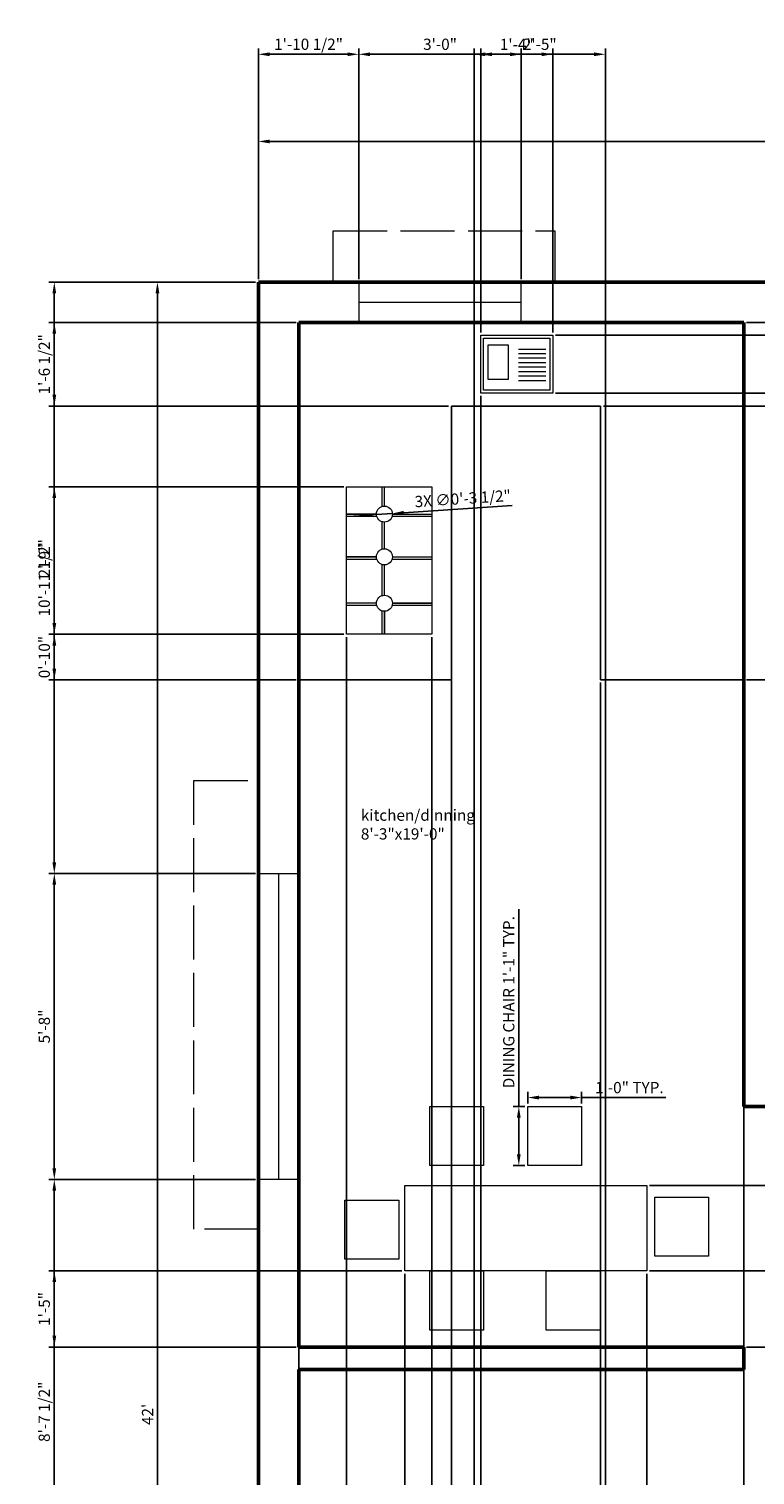
# Model space of a CAD drawing. Units: millimetres. Extents: x 3095 to 3505, y 1097 to 1734.
# Tile 4 of 5: x 3095 to 3256, y 1412 to 1734. Entities that reach past the tile are written whole.
import ezdxf

# ---------------------------------------------------------------- set-up
doc = ezdxf.new("R2010")
doc.units = ezdxf.units.MM
doc.linetypes.add('ACAD_ISO02W100', pattern=[15, 12, -3])
for name, color, linetype, lineweight, true_color in [('A-ANNO-DIMS', 32, 'Continuous', 18, 0xcd6928), ('A-AREA-IDEN', 152, 'Continuous', 18, 0x2776bb), ('A-EQPM', 9, 'Continuous', 18, 0xafd9aa), ('A-FLOR-CASE', 9, 'Continuous', 25, 0xafd9aa), ('A-FLOR-FIXT', 9, 'Continuous', 18, 0xafd9aa), ('A-FURN', 9, 'Continuous', 18, 0xafd9aa), ('A-GLAZ', 9, 'Continuous', 18, 0xd19cc7), ('A-ROOF-OVHD', 152, 'ACAD_ISO02W100', 13, 0x2776bb)]:
    doc.layers.add(name, color=color, linetype=linetype, lineweight=lineweight, true_color=true_color)
doc.layers.add('A-WALL', color=7, linetype='Continuous', lineweight=50)
doc.styles.get("Standard").update_dxf_attribs({"font": 'arial.ttf'})
doc.dimstyles.new('ISO-25', dxfattribs={"dimtxt": 2.5, "dimasz": 2.5, "dimexe": 1.25, "dimexo": 0.625, "dimtad": 1, "dimlunit": 3, "dimtxsty": 'Standard', "dimcen": 2.5, "dimadec": 0, "dimazin": 0, "dimtfac": 1, "dimtmove": 0, "dimatfit": 3, "dimfxl": 1, "dimarcsym": 0})

# ---------------------------------------------------------------- blocks, each defined once
blk = doc.blocks.new('*D10')
at = {"layer": 'A-ANNO-DIMS', "color": 0, "lineweight": -2, "transparency": 16777216}
for p, q in [((3145.86, 1677.94), (3145.86, 1709.87)), ((3457.86, 1677.94), (3457.86, 1709.87)), ((3148.36, 1708.62), (3455.36, 1708.62))]:
    blk.add_line(p, q, dxfattribs=at)
at = {"layer": 'A-ANNO-DIMS', "color": 0, "lineweight": 5, "transparency": 16777216}
for points in [[(3148.36, 1709.03), (3148.36, 1708.2), (3145.86, 1708.62)], [(3455.36, 1709.03), (3455.36, 1708.2), (3457.86, 1708.62)]]:
    blk.add_solid(points, dxfattribs=at)
at = {"layer": 'Defpoints', "color": 0, "lineweight": 5, "transparency": 16777216}
for p in [(3457.86, 1708.62), (3145.86, 1677.32), (3457.86, 1677.32)]:
    blk.add_point(p, dxfattribs=at)
at = {"layer": 'A-ANNO-DIMS', "color": 0, "transparency": 16777216, "insert": (3301.86, 1710.52), "char_height": 2.5, "attachment_point": 5}
blk.add_mtext("26'", dxfattribs=at)
blk = doc.blocks.new('*D11')
at = {"layer": 'A-ANNO-DIMS', "color": 0, "lineweight": -2, "transparency": 16777216}
for p, q in [((3145.24, 1677.32), (3122.17, 1677.32)), ((3123.42, 1674.82), (3123.42, 1175.82)), ((3145.24, 1173.32), (3122.17, 1173.32))]:
    blk.add_line(p, q, dxfattribs=at)
at = {"layer": 'A-ANNO-DIMS', "color": 0, "lineweight": 5, "transparency": 16777216}
for points in [[(3123, 1674.82), (3123.84, 1674.82), (3123.42, 1677.32)], [(3123, 1175.82), (3123.84, 1175.82), (3123.42, 1173.32)]]:
    blk.add_solid(points, dxfattribs=at)
at = {"layer": 'Defpoints', "color": 0, "lineweight": 5, "transparency": 16777216}
for p in [(3145.86, 1677.32), (3123.42, 1173.32), (3145.86, 1173.32)]:
    blk.add_point(p, dxfattribs=at)
at = {"layer": 'A-ANNO-DIMS', "color": 0, "transparency": 16777216, "insert": (3121.54, 1425.32), "char_height": 2.5, "attachment_point": 5, "rotation": 90}
blk.add_mtext("42'", dxfattribs=at)
blk = doc.blocks.new('CHAIR-DINING')
blk.add_lwpolyline([(0, 13.15), (12, 13.15), (12, 0), (0, 0)], close=True)
blk = doc.blocks.new('*D16')
at = {"layer": 'A-ANNO-DIMS', "color": 0, "lineweight": -2, "transparency": 16777216}
for p, q in [((3203.81, 1493.86), (3203.81, 1537.75)), ((3205.15, 1493.86), (3202.56, 1493.86)), ((3203.81, 1483.2), (3203.81, 1491.36)), ((3205.15, 1480.7), (3202.56, 1480.7))]:
    blk.add_line(p, q, dxfattribs=at)
at = {"layer": 'A-ANNO-DIMS', "color": 0, "lineweight": 5, "transparency": 16777216}
for points in [[(3203.39, 1491.36), (3204.22, 1491.36), (3203.81, 1493.86)], [(3203.39, 1483.2), (3204.22, 1483.2), (3203.81, 1480.7)]]:
    blk.add_solid(points, dxfattribs=at)
at = {"layer": 'Defpoints', "color": 0, "lineweight": 5, "transparency": 16777216}
for p in [(3203.81, 1493.86), (3205.78, 1493.86), (3205.78, 1480.7)]:
    blk.add_point(p, dxfattribs=at)
at = {"layer": 'A-ANNO-DIMS', "color": 0, "transparency": 16777216, "insert": (3201.89, 1517.06), "char_height": 2.5, "attachment_point": 5, "rotation": 90}
blk.add_mtext('DINING CHAIR 1\'-1" TYP.', dxfattribs=at)
blk = doc.blocks.new('*D17')
at = {"layer": 'A-ANNO-DIMS', "color": 0, "lineweight": -2, "transparency": 16777216}
for p, q in [((3205.78, 1494.48), (3205.78, 1497.08)), ((3217.78, 1494.48), (3217.78, 1497.08)), ((3208.28, 1495.83), (3215.28, 1495.83)), ((3217.78, 1495.83), (3236.53, 1495.83))]:
    blk.add_line(p, q, dxfattribs=at)
at = {"layer": 'A-ANNO-DIMS', "color": 0, "lineweight": 5, "transparency": 16777216}
for points in [[(3208.28, 1496.25), (3208.28, 1495.41), (3205.78, 1495.83)], [(3215.28, 1496.25), (3215.28, 1495.41), (3217.78, 1495.83)]]:
    blk.add_solid(points, dxfattribs=at)
at = {"layer": 'Defpoints', "color": 0, "lineweight": 5, "transparency": 16777216}
for p in [(3205.78, 1493.86), (3217.78, 1495.83), (3217.78, 1493.86)]:
    blk.add_point(p, dxfattribs=at)
at = {"layer": 'A-ANNO-DIMS', "color": 0, "transparency": 16777216, "insert": (3228.4, 1497.73), "char_height": 2.5, "attachment_point": 5}
blk.add_mtext('1\'-0" TYP.', dxfattribs=at)
blk = doc.blocks.new('*D30')
at = {"layer": 'A-ANNO-DIMS', "color": 0, "lineweight": -2, "transparency": 16777216}
for p, q in [((3145.86, 1677.94), (3145.86, 1729.27)), ((3168.2, 1677.94), (3168.2, 1729.27)), ((3148.36, 1728.02), (3165.7, 1728.02))]:
    blk.add_line(p, q, dxfattribs=at)
at = {"layer": 'A-ANNO-DIMS', "color": 0, "lineweight": 5, "transparency": 16777216}
for points in [[(3148.36, 1728.43), (3148.36, 1727.6), (3145.86, 1728.02)], [(3165.7, 1728.43), (3165.7, 1727.6), (3168.2, 1728.02)]]:
    blk.add_solid(points, dxfattribs=at)
at = {"layer": 'Defpoints', "color": 0, "lineweight": 5, "transparency": 16777216}
for p in [(3168.2, 1728.02), (3145.86, 1677.32), (3168.2, 1677.32)]:
    blk.add_point(p, dxfattribs=at)
at = {"layer": 'A-ANNO-DIMS', "color": 0, "transparency": 16777216, "insert": (3157.03, 1729.93), "char_height": 2.5, "attachment_point": 5}
blk.add_mtext('1\'-10 1/2"', dxfattribs=at)
blk = doc.blocks.new('*D31')
at = {"layer": 'A-ANNO-DIMS', "color": 0, "lineweight": -2, "transparency": 16777216}
for p, q in [((3168.2, 1677.94), (3168.2, 1729.27)), ((3204.36, 1677.94), (3204.36, 1729.27)), ((3170.7, 1728.02), (3201.86, 1728.02))]:
    blk.add_line(p, q, dxfattribs=at)
at = {"layer": 'A-ANNO-DIMS', "color": 0, "lineweight": 5, "transparency": 16777216}
for points in [[(3170.7, 1728.43), (3170.7, 1727.6), (3168.2, 1728.02)], [(3201.86, 1728.43), (3201.86, 1727.6), (3204.36, 1728.02)]]:
    blk.add_solid(points, dxfattribs=at)
at = {"layer": 'Defpoints', "color": 0, "lineweight": 5, "transparency": 16777216}
for p in [(3204.36, 1728.02), (3168.2, 1677.32), (3204.36, 1677.32)]:
    blk.add_point(p, dxfattribs=at)
at = {"layer": 'A-ANNO-DIMS', "color": 0, "transparency": 16777216, "insert": (3186.28, 1729.92), "char_height": 2.5, "attachment_point": 5}
blk.add_mtext('3\'-0"', dxfattribs=at)
blk = doc.blocks.new('*D34')
at = {"layer": 'A-ANNO-DIMS', "color": 0, "lineweight": -2, "transparency": 16777216}
for p, q in [((3145.24, 1677.32), (3099.22, 1677.32)), ((3100.47, 1674.82), (3100.47, 1548.2)), ((3145.24, 1545.7), (3099.22, 1545.7))]:
    blk.add_line(p, q, dxfattribs=at)
at = {"layer": 'A-ANNO-DIMS', "color": 0, "lineweight": 5, "transparency": 16777216}
for points in [[(3100.06, 1674.82), (3100.89, 1674.82), (3100.47, 1677.32)], [(3100.06, 1548.2), (3100.89, 1548.2), (3100.47, 1545.7)]]:
    blk.add_solid(points, dxfattribs=at)
at = {"layer": 'Defpoints', "color": 0, "lineweight": 5, "transparency": 16777216}
for p in [(3145.86, 1677.32), (3100.47, 1545.7), (3145.86, 1545.7)]:
    blk.add_point(p, dxfattribs=at)
at = {"layer": 'A-ANNO-DIMS', "color": 0, "transparency": 16777216, "insert": (3098.56, 1611.51), "char_height": 2.5, "attachment_point": 5, "rotation": 90}
blk.add_mtext('10\'-11 1/2"', dxfattribs=at)
blk = doc.blocks.new('*D35')
at = {"layer": 'A-ANNO-DIMS', "color": 0, "lineweight": -2, "transparency": 16777216}
for p, q in [((3145.24, 1545.7), (3099.22, 1545.7)), ((3100.47, 1543.2), (3100.47, 1480.1)), ((3145.24, 1477.6), (3099.22, 1477.6))]:
    blk.add_line(p, q, dxfattribs=at)
at = {"layer": 'A-ANNO-DIMS', "color": 0, "lineweight": 5, "transparency": 16777216}
for points in [[(3100.06, 1543.2), (3100.89, 1543.2), (3100.47, 1545.7)], [(3100.06, 1480.1), (3100.89, 1480.1), (3100.47, 1477.6)]]:
    blk.add_solid(points, dxfattribs=at)
at = {"layer": 'Defpoints', "color": 0, "lineweight": 5, "transparency": 16777216}
for p in [(3145.86, 1545.7), (3100.47, 1477.6), (3145.86, 1477.6)]:
    blk.add_point(p, dxfattribs=at)
at = {"layer": 'A-ANNO-DIMS', "color": 0, "transparency": 16777216, "insert": (3098.57, 1511.65), "char_height": 2.5, "attachment_point": 5, "rotation": 90}
blk.add_mtext('5\'-8"', dxfattribs=at)
blk = doc.blocks.new('*D36')
at = {"layer": 'A-ANNO-DIMS', "color": 0, "lineweight": -2, "transparency": 16777216}
for p, q in [((3145.24, 1477.6), (3099.22, 1477.6)), ((3100.47, 1475.1), (3100.47, 1376.7)), ((3145.24, 1374.2), (3099.22, 1374.2))]:
    blk.add_line(p, q, dxfattribs=at)
at = {"layer": 'A-ANNO-DIMS', "color": 0, "lineweight": 5, "transparency": 16777216}
for points in [[(3100.06, 1475.1), (3100.89, 1475.1), (3100.47, 1477.6)], [(3100.06, 1376.7), (3100.89, 1376.7), (3100.47, 1374.2)]]:
    blk.add_solid(points, dxfattribs=at)
at = {"layer": 'Defpoints', "color": 0, "lineweight": 5, "transparency": 16777216}
for p in [(3145.86, 1477.6), (3100.47, 1374.2), (3145.86, 1374.2)]:
    blk.add_point(p, dxfattribs=at)
at = {"layer": 'A-ANNO-DIMS', "color": 0, "transparency": 16777216, "insert": (3098.56, 1425.9), "char_height": 2.5, "attachment_point": 5, "rotation": 90}
blk.add_mtext('8\'-7 1/2"', dxfattribs=at)
blk = doc.blocks.new('*D48')
at = {"layer": 'A-ANNO-DIMS', "color": 0, "lineweight": -2, "transparency": 16777216}
for p, q in [((3254.49, 1668.32), (3504.29, 1668.32)), ((3503.04, 1665.82), (3503.04, 1591.3)), ((3254.49, 1588.8), (3504.29, 1588.8))]:
    blk.add_line(p, q, dxfattribs=at)
at = {"layer": 'A-ANNO-DIMS', "color": 0, "lineweight": 5, "transparency": 16777216}
for points in [[(3502.63, 1665.82), (3503.46, 1665.82), (3503.04, 1668.32)], [(3502.63, 1591.3), (3503.46, 1591.3), (3503.04, 1588.8)]]:
    blk.add_solid(points, dxfattribs=at)
at = {"layer": 'Defpoints', "color": 0, "lineweight": 5, "transparency": 16777216}
for p in [(3253.86, 1668.32), (3253.86, 1588.8), (3503.04, 1588.8)]:
    blk.add_point(p, dxfattribs=at)
at = {"layer": 'A-ANNO-DIMS', "color": 0, "transparency": 16777216, "insert": (3501.13, 1628.56), "char_height": 2.5, "attachment_point": 5, "rotation": 90}
blk.add_mtext('6\'-7 1/2"', dxfattribs=at)
blk = doc.blocks.new('*D49')
at = {"layer": 'A-ANNO-DIMS', "color": 0, "lineweight": -2, "transparency": 16777216}
for p, q in [((3154.86, 1588.17), (3154.86, 1134.75)), ((3188.81, 1588.17), (3188.81, 1134.75)), ((3157.36, 1136), (3186.31, 1136))]:
    blk.add_line(p, q, dxfattribs=at)
at = {"layer": 'A-ANNO-DIMS', "color": 0, "lineweight": 5, "transparency": 16777216}
for points in [[(3157.36, 1136.41), (3157.36, 1135.58), (3154.86, 1136)], [(3186.31, 1136.41), (3186.31, 1135.58), (3188.81, 1136)]]:
    blk.add_solid(points, dxfattribs=at)
at = {"layer": 'Defpoints', "color": 0, "lineweight": 5, "transparency": 16777216}
for p in [(3154.86, 1588.8), (3188.81, 1588.8), (3188.81, 1136)]:
    blk.add_point(p, dxfattribs=at)
at = {"layer": 'A-ANNO-DIMS', "color": 0, "transparency": 16777216, "insert": (3171.84, 1137.9), "char_height": 2.5, "attachment_point": 5}
blk.add_mtext('2\'-10"', dxfattribs=at)
blk = doc.blocks.new('*D50')
at = {"layer": 'A-ANNO-DIMS', "color": 0, "lineweight": -2, "transparency": 16777216}
for p, q in [((3222, 1588.17), (3222, 1134.75)), ((3253.86, 1588.17), (3253.86, 1134.75)), ((3224.5, 1136), (3251.36, 1136))]:
    blk.add_line(p, q, dxfattribs=at)
at = {"layer": 'A-ANNO-DIMS', "color": 0, "lineweight": 5, "transparency": 16777216}
for points in [[(3224.5, 1136.41), (3224.5, 1135.58), (3222, 1136)], [(3251.36, 1136.41), (3251.36, 1135.58), (3253.86, 1136)]]:
    blk.add_solid(points, dxfattribs=at)
at = {"layer": 'Defpoints', "color": 0, "lineweight": 5, "transparency": 16777216}
for p in [(3222, 1588.8), (3253.86, 1588.8), (3253.86, 1136)]:
    blk.add_point(p, dxfattribs=at)
at = {"layer": 'A-ANNO-DIMS', "color": 0, "transparency": 16777216, "insert": (3237.93, 1137.9), "char_height": 2.5, "attachment_point": 5}
blk.add_mtext('2\'-8"', dxfattribs=at)
blk = doc.blocks.new('*D51')
at = {"layer": 'A-ANNO-DIMS', "color": 0, "lineweight": -2, "transparency": 16777216}
for p, q in [((3154.24, 1668.32), (3099.22, 1668.32)), ((3100.47, 1652.23), (3100.47, 1665.82)), ((3188.18, 1649.73), (3099.22, 1649.73))]:
    blk.add_line(p, q, dxfattribs=at)
at = {"layer": 'A-ANNO-DIMS', "color": 0, "lineweight": 5, "transparency": 16777216}
for points in [[(3100.06, 1665.82), (3100.89, 1665.82), (3100.47, 1668.32)], [(3100.06, 1652.23), (3100.89, 1652.23), (3100.47, 1649.73)]]:
    blk.add_solid(points, dxfattribs=at)
at = {"layer": 'Defpoints', "color": 0, "lineweight": 5, "transparency": 16777216}
for p in [(3100.47, 1668.32), (3154.86, 1668.32), (3188.81, 1649.73)]:
    blk.add_point(p, dxfattribs=at)
at = {"layer": 'A-ANNO-DIMS', "color": 0, "transparency": 16777216, "insert": (3098.56, 1659.02), "char_height": 2.5, "attachment_point": 5, "rotation": 90}
blk.add_mtext('1\'-6 1/2"', dxfattribs=at)
blk = doc.blocks.new('*D52')
at = {"layer": 'A-ANNO-DIMS', "color": 0, "lineweight": -2, "transparency": 16777216}
for p, q in [((3178.42, 1456.63), (3178.42, 1134.75)), ((3232.26, 1456.63), (3232.26, 1134.75)), ((3180.92, 1136), (3229.76, 1136))]:
    blk.add_line(p, q, dxfattribs=at)
at = {"layer": 'A-ANNO-DIMS', "color": 0, "lineweight": 5, "transparency": 16777216}
for points in [[(3180.92, 1136.41), (3180.92, 1135.58), (3178.42, 1136)], [(3229.76, 1136.41), (3229.76, 1135.58), (3232.26, 1136)]]:
    blk.add_solid(points, dxfattribs=at)
at = {"layer": 'Defpoints', "color": 0, "lineweight": 5, "transparency": 16777216}
for p in [(3178.42, 1457.25), (3232.26, 1457.25), (3232.26, 1136)]:
    blk.add_point(p, dxfattribs=at)
at = {"layer": 'A-ANNO-DIMS', "color": 0, "transparency": 16777216, "insert": (3205.34, 1137.9), "char_height": 2.5, "attachment_point": 5}
blk.add_mtext('4\'-6"', dxfattribs=at)
blk = doc.blocks.new('*D53')
at = {"layer": 'A-ANNO-DIMS', "color": 0, "lineweight": -2, "transparency": 16777216}
for p, q in [((3232.89, 1476.25), (3504.29, 1476.25)), ((3503.04, 1473.75), (3503.04, 1459.75)), ((3232.89, 1457.25), (3504.29, 1457.25))]:
    blk.add_line(p, q, dxfattribs=at)
at = {"layer": 'A-ANNO-DIMS', "color": 0, "lineweight": 5, "transparency": 16777216}
for points in [[(3502.63, 1473.75), (3503.46, 1473.75), (3503.04, 1476.25)], [(3502.63, 1459.75), (3503.46, 1459.75), (3503.04, 1457.25)]]:
    blk.add_solid(points, dxfattribs=at)
at = {"layer": 'Defpoints', "color": 0, "lineweight": 5, "transparency": 16777216}
for p in [(3232.26, 1476.25), (3232.26, 1457.25), (3503.04, 1457.25)]:
    blk.add_point(p, dxfattribs=at)
at = {"layer": 'A-ANNO-DIMS', "color": 0, "transparency": 16777216, "insert": (3501.16, 1466.75), "char_height": 2.5, "attachment_point": 5, "rotation": 90}
blk.add_mtext('1\'-7"', dxfattribs=at)
blk = doc.blocks.new('*D54')
at = {"layer": 'A-ANNO-DIMS', "color": 0, "lineweight": -2, "transparency": 16777216}
for p, q in [((3254.49, 1493.86), (3504.29, 1493.86)), ((3503.04, 1491.36), (3503.04, 1442.82)), ((3254.49, 1440.32), (3504.29, 1440.32))]:
    blk.add_line(p, q, dxfattribs=at)
at = {"layer": 'A-ANNO-DIMS', "color": 0, "lineweight": 5, "transparency": 16777216}
for points in [[(3502.63, 1491.36), (3503.46, 1491.36), (3503.04, 1493.86)], [(3502.63, 1442.82), (3503.46, 1442.82), (3503.04, 1440.32)]]:
    blk.add_solid(points, dxfattribs=at)
at = {"layer": 'Defpoints', "color": 0, "lineweight": 5, "transparency": 16777216}
for p in [(3253.86, 1493.86), (3253.86, 1440.32), (3503.04, 1440.32)]:
    blk.add_point(p, dxfattribs=at)
at = {"layer": 'A-ANNO-DIMS', "color": 0, "transparency": 16777216, "insert": (3501.13, 1467.09), "char_height": 2.5, "attachment_point": 5, "rotation": 90}
blk.add_mtext('4\'-5 1/2"', dxfattribs=at)
blk = doc.blocks.new('*D55')
at = {"layer": 'A-ANNO-DIMS', "color": 0, "lineweight": -2, "transparency": 16777216}
for p, q in [((3195.33, 1666.1), (3195.33, 1729.27)), ((3211.36, 1666.1), (3211.36, 1729.27)), ((3197.83, 1728.02), (3208.86, 1728.02))]:
    blk.add_line(p, q, dxfattribs=at)
at = {"layer": 'A-ANNO-DIMS', "color": 0, "lineweight": 5, "transparency": 16777216}
for points in [[(3197.83, 1728.43), (3197.83, 1727.6), (3195.33, 1728.02)], [(3208.86, 1728.43), (3208.86, 1727.6), (3211.36, 1728.02)]]:
    blk.add_solid(points, dxfattribs=at)
at = {"layer": 'Defpoints', "color": 0, "lineweight": 5, "transparency": 16777216}
for p in [(3211.36, 1728.02), (3195.33, 1665.48), (3211.36, 1665.48)]:
    blk.add_point(p, dxfattribs=at)
at = {"layer": 'A-ANNO-DIMS', "color": 0, "transparency": 16777216, "insert": (3203.35, 1729.9), "char_height": 2.5, "attachment_point": 5}
blk.add_mtext('1\'-4"', dxfattribs=at)
blk = doc.blocks.new('*D56')
at = {"layer": 'A-ANNO-DIMS', "color": 0, "lineweight": -2, "transparency": 16777216}
for p, q in [((3211.99, 1665.48), (3504.29, 1665.48)), ((3503.04, 1662.98), (3503.04, 1655.1)), ((3211.99, 1652.6), (3504.29, 1652.6))]:
    blk.add_line(p, q, dxfattribs=at)
at = {"layer": 'A-ANNO-DIMS', "color": 0, "lineweight": 5, "transparency": 16777216}
for points in [[(3502.63, 1662.98), (3503.46, 1662.98), (3503.04, 1665.48)], [(3502.63, 1655.1), (3503.46, 1655.1), (3503.04, 1652.6)]]:
    blk.add_solid(points, dxfattribs=at)
at = {"layer": 'Defpoints', "color": 0, "lineweight": 5, "transparency": 16777216}
for p in [(3211.36, 1665.48), (3211.36, 1652.6), (3503.04, 1652.6)]:
    blk.add_point(p, dxfattribs=at)
at = {"layer": 'A-ANNO-DIMS', "color": 0, "transparency": 16777216, "insert": (3501.16, 1659.04), "char_height": 2.5, "attachment_point": 5, "rotation": 90}
blk.add_mtext('1\'-1"', dxfattribs=at)
blk = doc.blocks.new('*D57')
at = {"layer": 'A-ANNO-DIMS', "color": 0, "lineweight": -2, "transparency": 16777216}
for p, q in [((3165.47, 1598.31), (3165.47, 1134.75)), ((3184.42, 1598.31), (3184.42, 1134.75)), ((3167.97, 1136), (3181.92, 1136))]:
    blk.add_line(p, q, dxfattribs=at)
at = {"layer": 'A-ANNO-DIMS', "color": 0, "lineweight": 5, "transparency": 16777216}
for points in [[(3167.97, 1136.41), (3167.97, 1135.58), (3165.47, 1136)], [(3181.92, 1136.41), (3181.92, 1135.58), (3184.42, 1136)]]:
    blk.add_solid(points, dxfattribs=at)
at = {"layer": 'Defpoints', "color": 0, "lineweight": 5, "transparency": 16777216}
for p in [(3165.47, 1598.93), (3184.42, 1598.93), (3184.42, 1136)]:
    blk.add_point(p, dxfattribs=at)
at = {"layer": 'A-ANNO-DIMS', "color": 0, "transparency": 16777216, "insert": (3174.95, 1137.88), "char_height": 2.5, "attachment_point": 5}
blk.add_mtext('1\'-7"', dxfattribs=at)
blk = doc.blocks.new('*D58')
at = {"layer": 'A-ANNO-DIMS', "color": 0, "lineweight": -2, "transparency": 16777216}
for p, q in [((3164.85, 1631.75), (3099.22, 1631.75)), ((3100.47, 1629.25), (3100.47, 1601.43)), ((3164.85, 1598.93), (3099.22, 1598.93))]:
    blk.add_line(p, q, dxfattribs=at)
at = {"layer": 'A-ANNO-DIMS', "color": 0, "lineweight": 5, "transparency": 16777216}
for points in [[(3100.06, 1629.25), (3100.89, 1629.25), (3100.47, 1631.75)], [(3100.06, 1601.43), (3100.89, 1601.43), (3100.47, 1598.93)]]:
    blk.add_solid(points, dxfattribs=at)
at = {"layer": 'Defpoints', "color": 0, "lineweight": 5, "transparency": 16777216}
for p in [(3165.47, 1631.75), (3100.47, 1598.93), (3165.47, 1598.93)]:
    blk.add_point(p, dxfattribs=at)
at = {"layer": 'A-ANNO-DIMS', "color": 0, "transparency": 16777216, "insert": (3098.57, 1615.34), "char_height": 2.5, "attachment_point": 5, "rotation": 90}
blk.add_mtext('2\'-9"', dxfattribs=at)
blk = doc.blocks.new('*D65')
at = {"layer": 'A-ANNO-DIMS', "color": 0, "lineweight": -2, "transparency": 16777216}
for p, q in [((3178.42, 1456.63), (3178.42, 1134.75)), ((3154.86, 1439.69), (3154.86, 1134.75)), ((3175.92, 1136), (3157.36, 1136))]:
    blk.add_line(p, q, dxfattribs=at)
at = {"layer": 'A-ANNO-DIMS', "color": 0, "lineweight": 5, "transparency": 16777216}
for points in [[(3157.36, 1136.41), (3157.36, 1135.58), (3154.86, 1136)], [(3175.92, 1136.41), (3175.92, 1135.58), (3178.42, 1136)]]:
    blk.add_solid(points, dxfattribs=at)
at = {"layer": 'Defpoints', "color": 0, "lineweight": 5, "transparency": 16777216}
for p in [(3178.42, 1457.25), (3154.86, 1440.32), (3154.86, 1136)]:
    blk.add_point(p, dxfattribs=at)
at = {"layer": 'A-ANNO-DIMS', "color": 0, "transparency": 16777216, "insert": (3166.64, 1137.91), "char_height": 2.5, "attachment_point": 5}
blk.add_mtext('1\'-11 1/2"', dxfattribs=at)
blk = doc.blocks.new('*D66')
at = {"layer": 'A-ANNO-DIMS', "color": 0, "lineweight": -2, "transparency": 16777216}
for p, q in [((3177.8, 1457.25), (3099.22, 1457.25)), ((3100.47, 1454.75), (3100.47, 1442.82)), ((3154.24, 1440.32), (3099.22, 1440.32))]:
    blk.add_line(p, q, dxfattribs=at)
at = {"layer": 'A-ANNO-DIMS', "color": 0, "lineweight": 5, "transparency": 16777216}
for points in [[(3100.06, 1454.75), (3100.89, 1454.75), (3100.47, 1457.25)], [(3100.06, 1442.82), (3100.89, 1442.82), (3100.47, 1440.32)]]:
    blk.add_solid(points, dxfattribs=at)
at = {"layer": 'Defpoints', "color": 0, "lineweight": 5, "transparency": 16777216}
for p in [(3178.42, 1457.25), (3100.47, 1440.32), (3154.86, 1440.32)]:
    blk.add_point(p, dxfattribs=at)
at = {"layer": 'A-ANNO-DIMS', "color": 0, "transparency": 16777216, "insert": (3098.57, 1448.78), "char_height": 2.5, "attachment_point": 5, "rotation": 90}
blk.add_mtext('1\'-5"', dxfattribs=at)
blk = doc.blocks.new('*D70')
at = {"layer": 'A-ANNO-DIMS', "color": 0, "lineweight": -2, "transparency": 16777216}
for p, q in [((3165.47, 1598.31), (3165.47, 1134.75)), ((3154.86, 1588.17), (3154.86, 1134.75)), ((3157.36, 1136), (3162.97, 1136)), ((3165.47, 1136), (3183.64, 1136))]:
    blk.add_line(p, q, dxfattribs=at)
at = {"layer": 'A-ANNO-DIMS', "color": 0, "lineweight": 5, "transparency": 16777216}
for points in [[(3157.36, 1136.41), (3157.36, 1135.58), (3154.86, 1136)], [(3162.97, 1136.41), (3162.97, 1135.58), (3165.47, 1136)]]:
    blk.add_solid(points, dxfattribs=at)
at = {"layer": 'Defpoints', "color": 0, "lineweight": 5, "transparency": 16777216}
for p in [(3165.47, 1598.93), (3154.86, 1588.8), (3165.47, 1136)]:
    blk.add_point(p, dxfattribs=at)
at = {"layer": 'A-ANNO-DIMS', "color": 0, "transparency": 16777216, "insert": (3175.81, 1137.91), "char_height": 2.5, "attachment_point": 5}
blk.add_mtext('0\'-10 1/2"', dxfattribs=at)
blk = doc.blocks.new('*D71')
at = {"layer": 'A-ANNO-DIMS', "color": 0, "lineweight": -2, "transparency": 16777216}
for p, q in [((3164.85, 1598.93), (3099.22, 1598.93)), ((3100.47, 1591.3), (3100.47, 1596.43)), ((3154.24, 1588.8), (3099.22, 1588.8))]:
    blk.add_line(p, q, dxfattribs=at)
at = {"layer": 'A-ANNO-DIMS', "color": 0, "lineweight": 5, "transparency": 16777216}
for points in [[(3100.06, 1596.43), (3100.89, 1596.43), (3100.47, 1598.93)], [(3100.06, 1591.3), (3100.89, 1591.3), (3100.47, 1588.8)]]:
    blk.add_solid(points, dxfattribs=at)
at = {"layer": 'Defpoints', "color": 0, "lineweight": 5, "transparency": 16777216}
for p in [(3100.47, 1598.93), (3165.47, 1598.93), (3154.86, 1588.8)]:
    blk.add_point(p, dxfattribs=at)
at = {"layer": 'A-ANNO-DIMS', "color": 0, "transparency": 16777216, "insert": (3098.57, 1593.86), "char_height": 2.5, "attachment_point": 5, "rotation": 90}
blk.add_mtext('0\'-10"', dxfattribs=at)
blk = doc.blocks.new('*D72')
at = {"layer": 'A-ANNO-DIMS', "color": 0, "lineweight": -2, "transparency": 16777216}
for p, q in [((3195.33, 1651.97), (3195.33, 1134.75)), ((3188.81, 1649.1), (3188.81, 1134.75)), ((3188.81, 1136), (3172.59, 1136)), ((3192.83, 1136), (3191.31, 1136))]:
    blk.add_line(p, q, dxfattribs=at)
at = {"layer": 'A-ANNO-DIMS', "color": 0, "lineweight": 5, "transparency": 16777216}
for points in [[(3191.31, 1136.41), (3191.31, 1135.58), (3188.81, 1136)], [(3192.83, 1136.41), (3192.83, 1135.58), (3195.33, 1136)]]:
    blk.add_solid(points, dxfattribs=at)
at = {"layer": 'Defpoints', "color": 0, "lineweight": 5, "transparency": 16777216}
for p in [(3195.33, 1652.6), (3188.81, 1649.73), (3188.81, 1136)]:
    blk.add_point(p, dxfattribs=at)
at = {"layer": 'A-ANNO-DIMS', "color": 0, "transparency": 16777216, "insert": (3179.45, 1137.91), "char_height": 2.5, "attachment_point": 5}
blk.add_mtext('0\'-6 1/2"', dxfattribs=at)
blk = doc.blocks.new('*D73')
at = {"layer": 'A-ANNO-DIMS', "color": 0, "lineweight": -2, "transparency": 16777216}
for p, q in [((3503.04, 1655.1), (3503.04, 1657.6)), ((3211.99, 1652.6), (3504.29, 1652.6)), ((3503.04, 1652.6), (3503.04, 1649.73)), ((3222.62, 1649.73), (3504.29, 1649.73)), ((3503.04, 1647.23), (3503.04, 1636.83))]:
    blk.add_line(p, q, dxfattribs=at)
at = {"layer": 'A-ANNO-DIMS', "color": 0, "lineweight": 5, "transparency": 16777216}
for points in [[(3502.63, 1655.1), (3503.46, 1655.1), (3503.04, 1652.6)], [(3502.63, 1647.23), (3503.46, 1647.23), (3503.04, 1649.73)]]:
    blk.add_solid(points, dxfattribs=at)
at = {"layer": 'Defpoints', "color": 0, "lineweight": 5, "transparency": 16777216}
for p in [(3211.36, 1652.6), (3222, 1649.73), (3503.04, 1649.73)]:
    blk.add_point(p, dxfattribs=at)
at = {"layer": 'A-ANNO-DIMS', "color": 0, "transparency": 16777216, "insert": (3501.14, 1640.78), "char_height": 2.5, "attachment_point": 5, "rotation": 90}
blk.add_mtext('0\'-3"', dxfattribs=at)
blk = doc.blocks.new('*D76')
at = {"layer": 'A-ANNO-DIMS', "color": 0, "lineweight": -2, "transparency": 16777216}
for p, q in [((3193.86, 1347.34), (3193.86, 1729.27)), ((3223.06, 1333.89), (3223.06, 1729.27)), ((3196.36, 1728.02), (3220.56, 1728.02))]:
    blk.add_line(p, q, dxfattribs=at)
at = {"layer": 'A-ANNO-DIMS', "color": 0, "lineweight": 5, "transparency": 16777216}
for points in [[(3196.36, 1728.43), (3196.36, 1727.6), (3193.86, 1728.02)], [(3220.56, 1728.43), (3220.56, 1727.6), (3223.06, 1728.02)]]:
    blk.add_solid(points, dxfattribs=at)
at = {"layer": 'Defpoints', "color": 0, "lineweight": 5, "transparency": 16777216}
for p in [(3223.06, 1728.02), (3193.86, 1346.71), (3223.06, 1333.27)]:
    blk.add_point(p, dxfattribs=at)
at = {"layer": 'A-ANNO-DIMS', "color": 0, "transparency": 16777216, "insert": (3208.46, 1729.92), "char_height": 2.5, "attachment_point": 5}
blk.add_mtext('2\'-5"', dxfattribs=at)
blk = doc.blocks.new('*D88')
at = {"layer": 'A-ANNO-DIMS', "color": 0, "lineweight": -2, "transparency": 16777216}
for p, q in [((3169.64, 1625.41), (3167.14, 1625.25)), ((3172.13, 1625.58), (3175.69, 1625.81)), ((3202.31, 1627.57), (3178.18, 1625.98))]:
    blk.add_line(p, q, dxfattribs=at)
at = {"layer": 'A-ANNO-DIMS', "color": 0, "lineweight": 5, "transparency": 16777216}
for points in [[(3169.61, 1625.83), (3169.66, 1625), (3172.13, 1625.58)], [(3178.15, 1626.39), (3178.21, 1625.56), (3175.69, 1625.81)]]:
    blk.add_solid(points, dxfattribs=at)
at = {"layer": 'Defpoints', "color": 0, "lineweight": 5, "transparency": 16777216}
for p in [(3172.13, 1625.58), (3175.69, 1625.81)]:
    blk.add_point(p, dxfattribs=at)
at = {"layer": 'A-ANNO-DIMS', "color": 0, "transparency": 16777216, "insert": (3191.36, 1628.82), "char_height": 2.5, "attachment_point": 5, "rotation": 3.7821}
blk.add_mtext('3X ∅0\'-3 1/2"', dxfattribs=at)

msp = doc.modelspace()

# ---------------------------------------------------------------- linework, layer by layer
at = {"layer": 'A-EQPM'}
for p, q in [((3173.408, 1627.405), (3173.408, 1631.748)), ((3173.908, 1627.477), (3173.908, 1631.748)), ((3172.126, 1625.695), (3165.474, 1625.695)), ((3165.474, 1625.695), (3172.126, 1625.695)), ((3175.691, 1625.695), (3184.422, 1625.695)), ((3165.474, 1625.195), (3172.198, 1625.195)), ((3173.408, 1617.884), (3173.408, 1623.984)), ((3173.908, 1617.956), (3173.908, 1623.913)), ((3175.619, 1625.195), (3184.422, 1625.195)), ((3165.474, 1616.174), (3172.126, 1616.174)), ((3172.126, 1616.174), (3165.474, 1616.174)), ((3165.474, 1615.674), (3172.198, 1615.674)), ((3175.619, 1615.674), (3184.422, 1615.674)), ((3175.691, 1616.174), (3184.422, 1616.174)), ((3173.408, 1607.542), (3173.408, 1614.463)), ((3173.908, 1607.614), (3173.908, 1614.391)), ((3172.126, 1605.832), (3165.474, 1605.832)), ((3172.198, 1605.332), (3165.474, 1605.332)), ((3173.408, 1598.93), (3173.408, 1604.121)), ((3173.908, 1598.93), (3173.908, 1604.05)), ((3173.908, 1604.05), (3173.908, 1598.93)), ((3184.422, 1605.332), (3175.619, 1605.332)), ((3175.691, 1605.832), (3184.422, 1605.832)), ((3184.422, 1605.832), (3175.691, 1605.832))]:
    msp.add_line(p, q, dxfattribs=at)
msp.add_lwpolyline([(3165.474, 1631.748), (3184.422, 1631.748), (3184.422, 1598.93), (3165.474, 1598.93)], close=True, dxfattribs=at)
for centre in [(3173.908, 1625.695), (3173.908, 1616.174), (3173.908, 1605.832)]:
    msp.add_circle(centre, 1.782, dxfattribs=at)
at = {"layer": 'A-FLOR-CASE'}
for p, q in [((3188.808, 1588.796), (3188.808, 1649.727)), ((3188.808, 1649.727), (3221.995, 1649.727)), ((3221.995, 1649.727), (3221.995, 1588.796)), ((3154.862, 1588.796), (3188.808, 1588.796)), ((3221.995, 1588.796), (3253.862, 1588.796))]:
    msp.add_line(p, q, dxfattribs=at)
at = {"layer": 'A-FLOR-FIXT'}
for p, q in [((3203.74, 1662.426), (3209.842, 1662.426)), ((3203.74, 1661.426), (3209.842, 1661.426)), ((3203.74, 1660.426), (3209.842, 1660.426)), ((3203.74, 1659.426), (3209.842, 1659.426)), ((3203.74, 1658.426), (3209.842, 1658.426)), ((3203.74, 1657.426), (3209.842, 1657.426)), ((3203.74, 1656.426), (3209.842, 1656.426)), ((3203.74, 1655.426), (3209.842, 1655.426))]:
    msp.add_line(p, q, dxfattribs=at)
for points in [[(3195.33, 1665.476), (3211.364, 1665.476), (3211.364, 1652.599), (3195.33, 1652.599)], [(3195.978, 1664.828), (3210.715, 1664.828), (3210.715, 1653.248), (3195.978, 1653.248)], [(3197.018, 1663.35), (3201.463, 1663.35), (3201.463, 1655.651), (3197.018, 1655.651)]]:
    msp.add_lwpolyline(points, close=True, dxfattribs=at)
at = {"layer": 'A-FURN'}
msp.add_lwpolyline([(3178.42, 1476.252), (3232.262, 1476.252), (3232.262, 1457.251), (3178.42, 1457.251)], close=True, dxfattribs=at)
at = {"layer": 'A-GLAZ'}
for p, q in [((3168.199, 1677.316), (3168.199, 1668.316)), ((3204.362, 1677.316), (3168.199, 1677.316)), ((3168.199, 1677.316), (3168.199, 1672.816)), ((3204.362, 1668.316), (3204.362, 1677.316)), ((3168.199, 1672.816), (3204.362, 1672.816)), ((3168.199, 1668.316), (3204.362, 1668.316)), ((3145.862, 1545.701), (3154.862, 1545.701)), ((3145.862, 1477.599), (3145.862, 1545.701)), ((3145.862, 1545.701), (3150.362, 1545.701)), ((3150.362, 1545.701), (3150.362, 1477.599)), ((3154.862, 1545.701), (3154.862, 1477.599)), ((3154.862, 1477.599), (3145.862, 1477.599))]:
    msp.add_line(p, q, dxfattribs=at)
at = {"layer": 'A-ROOF-OVHD'}
for p, q in [((3162.523, 1677.316), (3162.523, 1688.729)), ((3162.523, 1688.729), (3211.855, 1688.729)), ((3211.855, 1688.729), (3211.855, 1677.316)), ((3131.524, 1466.565), (3131.524, 1566.424)), ((3131.524, 1566.424), (3145.862, 1566.424)), ((3145.862, 1466.565), (3131.524, 1466.565))]:
    msp.add_line(p, q, dxfattribs=at)
at = {"layer": 'A-WALL'}
for p, q in [((3145.862, 1677.316), (3457.862, 1677.316)), ((3145.862, 1173.316), (3145.862, 1677.316)), ((3154.862, 1668.316), (3253.862, 1668.316)), ((3154.862, 1440.316), (3154.862, 1668.316)), ((3253.862, 1493.863), (3253.862, 1668.316)), ((3253.862, 1493.863), (3258.862, 1493.863)), ((3154.862, 1440.316), (3253.862, 1440.316)), ((3253.862, 1440.316), (3253.862, 1435.316)), ((3154.862, 1435.316), (3253.862, 1435.316)), ((3154.862, 1259.316), (3154.862, 1435.316))]:
    msp.add_line(p, q, dxfattribs=at)

# ---------------------------------------------------------------- block references
at = {"layer": 'A-FURN'}
for p in [(3183.985, 1480.704), (3205.779, 1480.704), (3165.083, 1459.883), (3234.029, 1460.527), (3183.985, 1444.098), (3209.876, 1444.098)]:
    msp.add_blockref('CHAIR-DINING', p, dxfattribs=at)

# ---------------------------------------------------------------- texts
at = {"layer": 'A-AREA-IDEN', "insert": (3168.665, 1559.93), "char_height": 2.5, "attachment_point": 1}
msp.add_mtext_dynamic_manual_height_columns('kitchen/dinning\\P8\'-3"x19\'-0"', width=72.24911, gutter_width=12.5, heights=[0], dxfattribs=at)

# ---------------------------------------------------------------- dimensions: what is measured, and where the dimension line sits
at = {"layer": 'A-ANNO-DIMS'}
for base, p1, p2, override, picture, middle in [((3168.199, 1728.017), (3145.862, 1677.316), (3168.199, 1677.316), {"dimdec": 1, "dimlfac": 1, "dimrnd": 0, "dimzin": 1, "dimdsep": 46, "dimlunit": 4, "dimfrac": 2}, '*D30', (3157.031, 1729.935)), ((3204.362, 1728.017), (3168.199, 1677.316), (3204.362, 1677.316), {"dimdec": 1, "dimlfac": 1, "dimrnd": 0, "dimzin": 1, "dimdsep": 46, "dimlunit": 4, "dimfrac": 2}, '*D31', (3186.281, 1729.92)), ((3223.059, 1728.017), (3193.862, 1346.711), (3223.059, 1333.27), {"dimdec": 1, "dimlfac": 1, "dimrnd": 0, "dimzin": 1, "dimdsep": 46, "dimlunit": 4, "dimfrac": 2}, '*D76', (3208.461, 1729.919)), ((3211.364, 1728.017), (3195.33, 1665.476), (3211.364, 1665.476), {"dimdec": 1, "dimlfac": 1, "dimrnd": 0, "dimzin": 1, "dimdsep": 46, "dimlunit": 4, "dimfrac": 2}, '*D55', (3203.347, 1729.897)), ((3457.862, 1708.616), (3145.862, 1677.316), (3457.862, 1677.316), {"dimclrd": 0, "dimclre": 0, "dimclrt": 0}, '*D10', (3301.862, 1710.518)), ((3188.808, 1135.996), (3195.33, 1652.599), (3188.808, 1649.727), {"dimdec": 1, "dimlfac": 1, "dimrnd": 0, "dimzin": 1, "dimdsep": 46, "dimlunit": 4, "dimfrac": 2}, '*D72', (3179.447, 1137.914)), ((3165.474, 1135.996), (3154.862, 1588.796), (3165.474, 1598.93), {"dimdec": 1, "dimlfac": 1, "dimrnd": 0, "dimzin": 1, "dimdsep": 46, "dimlunit": 4, "dimfrac": 2}, '*D70', (3175.806, 1137.914)), ((3184.422, 1135.996), (3165.474, 1598.93), (3184.422, 1598.93), {"dimdec": 1, "dimlfac": 1, "dimrnd": 0, "dimzin": 1, "dimdsep": 46, "dimlunit": 4, "dimfrac": 2}, '*D57', (3174.948, 1137.877)), ((3188.808, 1135.996), (3154.862, 1588.796), (3188.808, 1588.796), {"dimdec": 1, "dimlfac": 1, "dimrnd": 0, "dimzin": 1, "dimdsep": 46, "dimlunit": 4, "dimfrac": 2}, '*D49', (3171.835, 1137.898)), ((3253.862, 1135.996), (3221.995, 1588.796), (3253.862, 1588.796), {"dimdec": 1, "dimlfac": 1, "dimrnd": 0, "dimzin": 1, "dimdsep": 46, "dimlunit": 4, "dimfrac": 2}, '*D50', (3237.929, 1137.898)), ((3154.862, 1135.996), (3178.42, 1457.251), (3154.862, 1440.316), {"dimdec": 1, "dimlfac": 1, "dimrnd": 0, "dimzin": 1, "dimdsep": 46, "dimlunit": 4, "dimfrac": 2}, '*D65', (3166.641, 1137.914)), ((3232.262, 1135.996), (3178.42, 1457.251), (3232.262, 1457.251), {"dimdec": 1, "dimlfac": 1, "dimrnd": 0, "dimzin": 1, "dimdsep": 46, "dimlunit": 4, "dimfrac": 2}, '*D52', (3205.341, 1137.898))]:
    dim = msp.add_linear_dim(base=base, p1=p1, p2=p2, dimstyle='ISO-25', override=override, dxfattribs=at)
    dim.commit()
    dim.dimension.update_dxf_attribs({"geometry": picture, "text_midpoint": middle})
for base, p1, p2, override, picture, middle in [((3100.474, 1545.701), (3145.862, 1677.316), (3145.862, 1545.701), {"dimdec": 1, "dimlfac": 1, "dimrnd": 0, "dimzin": 1, "dimdsep": 46, "dimlunit": 4, "dimfrac": 2}, '*D34', (3098.556, 1611.509)), ((3123.421, 1173.316), (3145.862, 1677.316), (3145.862, 1173.316), {"dimclrd": 0, "dimclre": 0, "dimclrt": 0}, '*D11', (3121.541, 1425.316)), ((3100.474, 1668.316), (3188.808, 1649.727), (3154.862, 1668.316), {"dimdec": 1, "dimlfac": 1, "dimrnd": 0, "dimzin": 1, "dimdsep": 46, "dimlunit": 4, "dimfrac": 2}, '*D51', (3098.556, 1659.022)), ((3503.043, 1588.796), (3253.862, 1668.316), (3253.862, 1588.796), {"dimdec": 1, "dimlfac": 1, "dimrnd": 0, "dimzin": 1, "dimdsep": 46, "dimlunit": 4, "dimfrac": 2}, '*D48', (3501.125, 1628.556)), ((3503.043, 1652.599), (3211.364, 1665.476), (3211.364, 1652.599), {"dimdec": 1, "dimlfac": 1, "dimrnd": 0, "dimzin": 1, "dimdsep": 46, "dimlunit": 4, "dimfrac": 2}, '*D56', (3501.163, 1659.038)), ((3503.043, 1649.727), (3211.364, 1652.599), (3221.995, 1649.727), {"dimdec": 1, "dimlfac": 1, "dimrnd": 0, "dimzin": 1, "dimdsep": 46, "dimlunit": 4, "dimfrac": 2}, '*D73', (3501.141, 1640.78)), ((3100.474, 1598.93), (3165.474, 1631.748), (3165.474, 1598.93), {"dimdec": 1, "dimlfac": 1, "dimrnd": 0, "dimzin": 1, "dimdsep": 46, "dimlunit": 4, "dimfrac": 2}, '*D58', (3098.572, 1615.339)), ((3100.474, 1598.93), (3154.862, 1588.796), (3165.474, 1598.93), {"dimdec": 1, "dimlfac": 1, "dimrnd": 0, "dimzin": 1, "dimdsep": 46, "dimlunit": 4, "dimfrac": 2}, '*D71', (3098.572, 1593.863)), ((3100.474, 1477.599), (3145.862, 1545.701), (3145.862, 1477.599), {"dimdec": 1, "dimlfac": 1, "dimrnd": 0, "dimzin": 1, "dimdsep": 46, "dimlunit": 4, "dimfrac": 2}, '*D35', (3098.572, 1511.65)), ((3503.043, 1440.316), (3253.862, 1493.863), (3253.862, 1440.316), {"dimdec": 1, "dimlfac": 1, "dimrnd": 0, "dimzin": 1, "dimdsep": 46, "dimlunit": 4, "dimfrac": 2}, '*D54', (3501.125, 1467.09)), ((3100.474, 1374.196), (3145.862, 1477.599), (3145.862, 1374.196), {"dimdec": 1, "dimlfac": 1, "dimrnd": 0, "dimzin": 1, "dimdsep": 46, "dimlunit": 4, "dimfrac": 2}, '*D36', (3098.556, 1425.897)), ((3503.043, 1457.251), (3232.262, 1476.252), (3232.262, 1457.251), {"dimdec": 1, "dimlfac": 1, "dimrnd": 0, "dimzin": 1, "dimdsep": 46, "dimlunit": 4, "dimfrac": 2}, '*D53', (3501.163, 1466.752)), ((3100.474, 1440.316), (3178.42, 1457.251), (3154.862, 1440.316), {"dimdec": 1, "dimlfac": 1, "dimrnd": 0, "dimzin": 1, "dimdsep": 46, "dimlunit": 4, "dimfrac": 2}, '*D66', (3098.572, 1448.784))]:
    dim = msp.add_linear_dim(base=base, p1=p1, p2=p2, angle=90, dimstyle='ISO-25', override=override, dxfattribs=at)
    dim.commit()
    dim.dimension.update_dxf_attribs({"geometry": picture, "text_midpoint": middle})
dim = msp.add_diameter_dim_2p(p1=(3172.13, 1625.577), p2=(3175.687, 1625.812), text='3X <>', dimstyle='ISO-25', override={"dimdec": 1, "dimlfac": 1, "dimrnd": 0, "dimzin": 1, "dimdsep": 46, "dimlunit": 4, "dimfrac": 2}, dxfattribs=at)
dim.commit()
dim.dimension.update_dxf_attribs({"geometry": '*D88', "text_midpoint": (3191.491, 1626.857), "dimtype": 163})
dim = msp.add_linear_dim(base=(3203.807, 1493.858), p1=(3205.78, 1480.704), p2=(3205.78, 1493.858), angle=90, text='DINING CHAIR <> TYP.', dimstyle='ISO-25', override={"dimdec": 1, "dimlfac": 1, "dimrnd": 0, "dimzin": 1, "dimdsep": 46, "dimlunit": 4, "dimfrac": 2}, dxfattribs=at)
dim.commit()
dim.dimension.update_dxf_attribs({"geometry": '*D16', "text_midpoint": (3201.889, 1517.055)})
dim = msp.add_linear_dim(base=(3217.777, 1495.831), p1=(3205.78, 1493.858), p2=(3217.777, 1493.858), text='<> TYP.', dimstyle='ISO-25', override={"dimdec": 1, "dimlfac": 1, "dimrnd": 0, "dimzin": 1, "dimdsep": 46, "dimlunit": 4, "dimfrac": 2}, dxfattribs=at)
dim.commit()
dim.dimension.update_dxf_attribs({"geometry": '*D17', "text_midpoint": (3228.404, 1497.732)})

doc.saveas('drawing.dxf')
